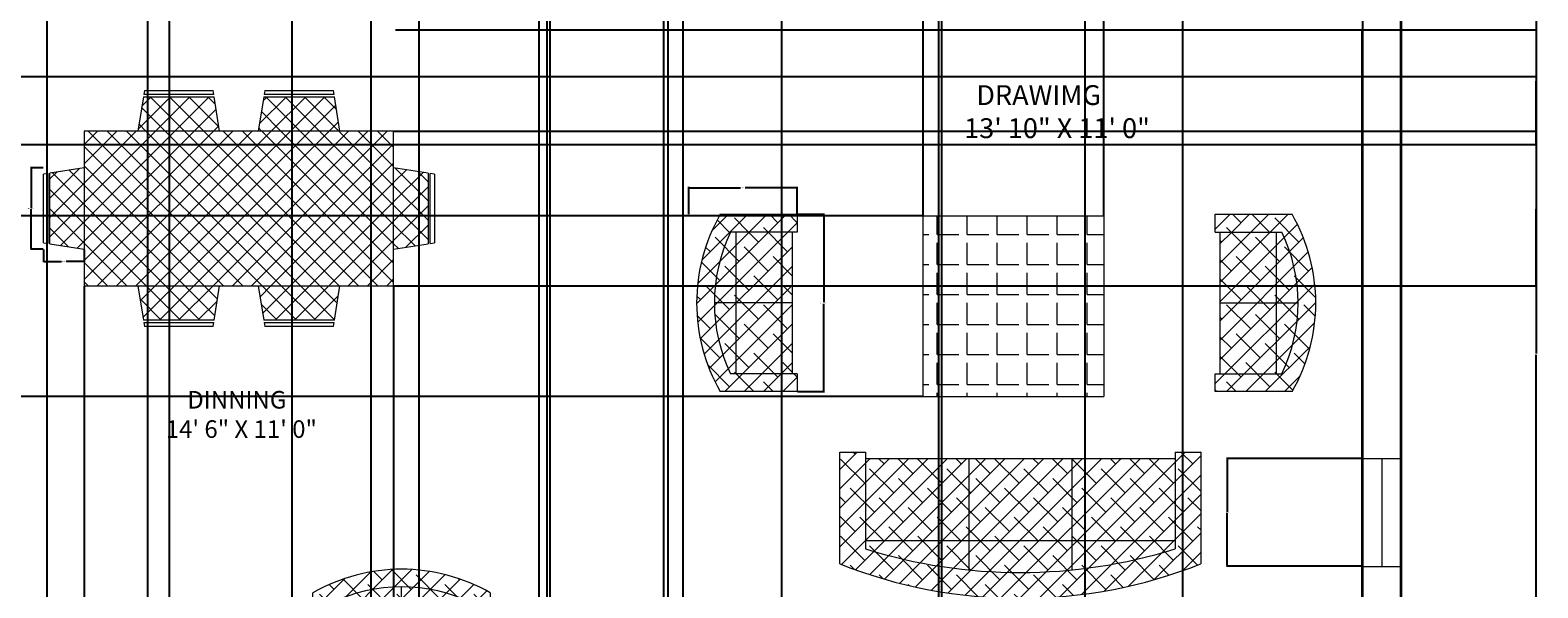
# Model space of a CAD drawing. Units: inches. Extents: x 2284228 to 3635239, y 3024422 to 8351872.
# Tile 4 of 7: x 3634888 to 3635239, y 8351470 to 8351600. Entities that reach past the tile are written whole.
import ezdxf

# ---------------------------------------------------------------- set-up
doc = ezdxf.new("R2010")
doc.units = ezdxf.units.IN
for name, color, linetype, lineweight in [('A-ANNO-DIMS', 2, 'Continuous', 18), ('A-AREA-IDEN', 7, 'Continuous', 18), ('A-FURN', 8, 'Continuous', 18), ('A-FURN-PATT', 9, 'Continuous', 13), ('A-GLAZ', 4, 'Continuous', 18), ('A-WALL', 7, 'Continuous', 35)]:
    doc.layers.add(name, color=color, linetype=linetype, lineweight=lineweight)
doc.styles.get("Standard").update_dxf_attribs({"font": 'arial.ttf'})
doc.dimstyles.get("Standard").update_dxf_attribs({"dimtxt": 0.18, "dimasz": 0.18, "dimexe": 0.18, "dimexo": 0.0625, "dimgap": 0.09, "dimtad": 0, "dimtih": 1, "dimtoh": 1, "dimdec": 4, "dimzin": 0, "dimdsep": 46, "dimtxsty": 'Standard', "dimcen": 0.09, "dimadec": 0, "dimazin": 0, "dimtfac": 1, "dimtdec": 4, "dimtofl": 0, "dimtmove": 0, "dimatfit": 3, "dimfxl": 1, "dimtolj": 1, "dimtzin": 0, "dimarcsym": 0})

# ---------------------------------------------------------------- blocks, each defined once
blk = doc.blocks.new('Sofa - Roundback 7 ft.')
for p, q in [((-12.00002, -32.4421), (-12.00003, -6.5971)), ((11.99997, -32.4421), (11.99998, -6.5971)), ((-36.000027, -34), (-36.000027, -11.4696)), ((-35.999844, -13.3819), (35.9998, -13.3819)), ((35.99998, -34), (35.99998, -11.4696)), ((-36.000027, -32.4421), (35.99998, -32.4421))]:
    blk.add_line(p, q)
for points in [[(-36.000027, -34), (-42.000027, -34), (-42.000027, -8)], [(41.99998, -8), (41.99998, -34), (35.99998, -34)]]:
    blk.add_lwpolyline(points)
for centre, radius, start, end in [((0, -114.25), 114.25, 68.43141, 111.5686), ((-0.00001, -127.1968), 121.1968, 72.72033, 107.2797)]:
    blk.add_arc(centre, radius, start, end)
blk = doc.blocks.new('Sofa - Roundback Loveseat 5 ft.')
for p, q in [((0, -32.44198), (0, -5.99998)), ((-24, -33.99998), (-24, -11.46958)), ((-23.9998, -13.38178), (23.99986, -13.38178)), ((24.00004, -33.99998), (24.00004, -11.46958)), ((-24, -32.44198), (24.00004, -32.44198))]:
    blk.add_line(p, q)
for points in [[(-24, -33.99998), (-30, -33.99998), (-30, -7.99998)], [(30.00004, -7.99998), (30.00004, -33.99998), (24.00004, -33.99998)]]:
    blk.add_lwpolyline(points)
for centre, radius, start, end in [((0, -60.24998), 60.24998, 60.13715, 119.8628), ((0, -61.38438), 55.38444, 64.32083, 115.6792)]:
    blk.add_arc(centre, radius, start, end)
blk = doc.blocks.new('CHAIR-DINING')
for p, q in [((1.25, 8), (0, 0)), ((1.25, 8), (17.72, 8)), ((1.48, 9.5), (1.33, 8.5)), ((17.64, 8.5), (1.33, 8.5)), ((1.48, 9.5), (17.48, 9.5)), ((17.64, 8.5), (17.48, 9.5)), ((18.97, 0), (17.72, 8))]:
    blk.add_line(p, q)
blk = doc.blocks.new('*D24')
at = {"layer": 'A-ANNO-DIMS', "color": 0, "lineweight": -2, "transparency": 16777216}
for p, q in [((3635066.29, 8351557.1), (3635072.6, 8351557.1)), ((3635072.42, 8351556.92), (3635072.42, 8351536.66)), ((3635072.42, 8351516.02), (3635072.42, 8351536.29)), ((3635066.29, 8351515.84), (3635072.6, 8351515.84))]:
    blk.add_line(p, q, dxfattribs=at)
at = {"layer": 'A-ANNO-DIMS', "color": 0, "transparency": 16777216}
for points in [[(3635072.39, 8351556.92), (3635072.45, 8351556.92), (3635072.42, 8351557.1)], [(3635072.39, 8351516.02), (3635072.45, 8351516.02), (3635072.42, 8351515.84)]]:
    blk.add_solid(points, dxfattribs=at)
at = {"layer": 'Defpoints', "color": 0, "transparency": 16777216}
for p in [(3635066.23, 8351557.1), (3635072.42, 8351557.1), (3635066.23, 8351515.84)]:
    blk.add_point(p, dxfattribs=at)
at = {"layer": 'A-ANNO-DIMS', "color": 0, "transparency": 16777216, "insert": (3635072.42, 8351536.47), "char_height": 0.18, "attachment_point": 5}
blk.add_mtext('\\A1;LOVESEAT 41 TYP.', dxfattribs=at)
blk = doc.blocks.new('*D25')
at = {"layer": 'A-ANNO-DIMS', "color": 0, "lineweight": -2, "transparency": 16777216}
for p, q in [((3635041.02, 8351557.16), (3635041.02, 8351563.47)), ((3635041.2, 8351563.29), (3635053.09, 8351563.29)), ((3635066.05, 8351563.29), (3635054.15, 8351563.29)), ((3635066.23, 8351557.16), (3635066.23, 8351563.47))]:
    blk.add_line(p, q, dxfattribs=at)
at = {"layer": 'A-ANNO-DIMS', "color": 0, "transparency": 16777216}
for points in [[(3635041.2, 8351563.32), (3635041.2, 8351563.26), (3635041.02, 8351563.29)], [(3635066.05, 8351563.32), (3635066.05, 8351563.26), (3635066.23, 8351563.29)]]:
    blk.add_solid(points, dxfattribs=at)
at = {"layer": 'Defpoints', "color": 0, "transparency": 16777216}
for p in [(3635041.02, 8351563.29), (3635041.02, 8351557.1), (3635066.23, 8351557.1)]:
    blk.add_point(p, dxfattribs=at)
at = {"layer": 'A-ANNO-DIMS', "color": 0, "transparency": 16777216, "insert": (3635053.62, 8351563.29), "char_height": 0.18, "attachment_point": 5}
blk.add_mtext('\\A1;25 TYP.', dxfattribs=at)
blk = doc.blocks.new('*D26')
at = {"layer": 'A-ANNO-DIMS', "color": 0, "lineweight": -2, "transparency": 16777216}
for p, q in [((3634890.78, 8351567.93), (3634887.82, 8351567.93)), ((3634888, 8351567.75), (3634888, 8351558.63)), ((3634888, 8351549.14), (3634888, 8351558.27)), ((3634890.79, 8351548.96), (3634887.82, 8351548.96))]:
    blk.add_line(p, q, dxfattribs=at)
at = {"layer": 'A-ANNO-DIMS', "color": 0, "transparency": 16777216}
for points in [[(3634888.03, 8351567.75), (3634887.97, 8351567.75), (3634888, 8351567.93)], [(3634888.03, 8351549.14), (3634887.97, 8351549.14), (3634888, 8351548.96)]]:
    blk.add_solid(points, dxfattribs=at)
at = {"layer": 'Defpoints', "color": 0, "transparency": 16777216}
for p in [(3634888, 8351567.93), (3634890.85, 8351567.93), (3634890.85, 8351548.96)]:
    blk.add_point(p, dxfattribs=at)
at = {"layer": 'A-ANNO-DIMS', "color": 0, "transparency": 16777216, "insert": (3634888, 8351558.45), "char_height": 0.18, "attachment_point": 5}
blk.add_mtext('\\A1;CHAIR 19 TYP.', dxfattribs=at)
blk = doc.blocks.new('*D27')
at = {"layer": 'A-ANNO-DIMS', "color": 0, "lineweight": -2, "transparency": 16777216}
for p, q in [((3634890.85, 8351548.9), (3634890.85, 8351545.94)), ((3634900.35, 8351548.9), (3634900.35, 8351545.94)), ((3634891.03, 8351546.12), (3634895.08, 8351546.12)), ((3634900.17, 8351546.12), (3634896.12, 8351546.12))]:
    blk.add_line(p, q, dxfattribs=at)
at = {"layer": 'A-ANNO-DIMS', "color": 0, "transparency": 16777216}
for points in [[(3634891.03, 8351546.15), (3634891.03, 8351546.09), (3634890.85, 8351546.12)], [(3634900.17, 8351546.15), (3634900.17, 8351546.09), (3634900.35, 8351546.12)]]:
    blk.add_solid(points, dxfattribs=at)
at = {"layer": 'Defpoints', "color": 0, "transparency": 16777216}
for p in [(3634890.85, 8351548.96), (3634900.35, 8351548.97), (3634890.85, 8351546.12)]:
    blk.add_point(p, dxfattribs=at)
at = {"layer": 'A-ANNO-DIMS', "color": 0, "transparency": 16777216, "insert": (3634895.6, 8351546.12), "char_height": 0.18, "attachment_point": 5}
blk.add_mtext('\\A1;10 TYP.', dxfattribs=at)
blk = doc.blocks.new('*D41')
at = {"layer": 'A-ANNO-DIMS', "color": 0, "lineweight": -2, "transparency": 16777216}
for p, q in [((3635053.81, 8351799.01), (3635238.38, 8351799.01)), ((3635238.2, 8351798.83), (3635238.2, 8351524.72)), ((3635238.2, 8351250.24), (3635238.2, 8351524.36)), ((3635039.81, 8351250.06), (3635238.38, 8351250.06))]:
    blk.add_line(p, q, dxfattribs=at)
at = {"layer": 'A-ANNO-DIMS', "color": 0, "transparency": 16777216}
for points in [[(3635238.17, 8351798.83), (3635238.23, 8351798.83), (3635238.2, 8351799.01)], [(3635238.17, 8351250.24), (3635238.23, 8351250.24), (3635238.2, 8351250.06)]]:
    blk.add_solid(points, dxfattribs=at)
at = {"layer": 'Defpoints', "color": 0, "transparency": 16777216}
for p in [(3635053.75, 8351799.01), (3635238.2, 8351799.01), (3635039.75, 8351250.06)]:
    blk.add_point(p, dxfattribs=at)
at = {"layer": 'A-ANNO-DIMS', "color": 0, "transparency": 16777216, "insert": (3635238.2, 8351524.54), "char_height": 0.18, "attachment_point": 5}
blk.add_mtext('\\A1;549', dxfattribs=at)
blk = doc.blocks.new('*D49')
at = {"layer": 'A-ANNO-DIMS', "color": 0, "lineweight": -2, "transparency": 16777216}
for p, q in [((3634891.75, 8351310.63), (3634891.75, 8351830.64)), ((3634891.93, 8351830.46), (3634965.47, 8351830.46)), ((3635039.57, 8351830.46), (3634966.03, 8351830.46)), ((3635039.75, 8351310.63), (3635039.75, 8351830.64))]:
    blk.add_line(p, q, dxfattribs=at)
at = {"layer": 'A-ANNO-DIMS', "color": 0, "transparency": 16777216}
for points in [[(3634891.93, 8351830.49), (3634891.93, 8351830.43), (3634891.75, 8351830.46)], [(3635039.57, 8351830.49), (3635039.57, 8351830.43), (3635039.75, 8351830.46)]]:
    blk.add_solid(points, dxfattribs=at)
at = {"layer": 'Defpoints', "color": 0, "transparency": 16777216}
for p in [(3635039.75, 8351830.46), (3634891.75, 8351310.56), (3635039.75, 8351310.56)]:
    blk.add_point(p, dxfattribs=at)
at = {"layer": 'A-ANNO-DIMS', "color": 0, "transparency": 16777216, "insert": (3634965.75, 8351830.46), "char_height": 0.18, "attachment_point": 5}
blk.add_mtext('\\A1;148', dxfattribs=at)
blk = doc.blocks.new('*D52')
at = {"layer": 'A-ANNO-DIMS', "color": 0, "lineweight": -2, "transparency": 16777216}
for p, q in [((3635099.83, 8351748.5), (3635099.83, 8351218.43)), ((3635155.88, 8351748.5), (3635155.88, 8351218.43)), ((3635100.01, 8351218.61), (3635127.46, 8351218.61)), ((3635155.7, 8351218.61), (3635128.25, 8351218.61))]:
    blk.add_line(p, q, dxfattribs=at)
at = {"layer": 'A-ANNO-DIMS', "color": 0, "transparency": 16777216}
for points in [[(3635100.01, 8351218.64), (3635100.01, 8351218.58), (3635099.83, 8351218.61)], [(3635155.7, 8351218.64), (3635155.7, 8351218.58), (3635155.88, 8351218.61)]]:
    blk.add_solid(points, dxfattribs=at)
at = {"layer": 'Defpoints', "color": 0, "transparency": 16777216}
for p in [(3635099.83, 8351748.56), (3635155.88, 8351748.56), (3635155.88, 8351218.61)]:
    blk.add_point(p, dxfattribs=at)
at = {"layer": 'A-ANNO-DIMS', "color": 0, "transparency": 16777216, "insert": (3635127.85, 8351218.61), "char_height": 0.18, "attachment_point": 5}
blk.add_mtext('\\A1;56.06', dxfattribs=at)
blk = doc.blocks.new('*D53')
at = {"layer": 'A-ANNO-DIMS', "color": 0, "lineweight": -2, "transparency": 16777216}
for p, q in [((3635155.88, 8351748.5), (3635155.88, 8351218.43)), ((3635197.75, 8351748.5), (3635197.75, 8351218.43)), ((3635156.06, 8351218.61), (3635176.42, 8351218.61)), ((3635197.57, 8351218.61), (3635177.21, 8351218.61))]:
    blk.add_line(p, q, dxfattribs=at)
at = {"layer": 'A-ANNO-DIMS', "color": 0, "transparency": 16777216}
for points in [[(3635156.06, 8351218.64), (3635156.06, 8351218.58), (3635155.88, 8351218.61)], [(3635197.57, 8351218.64), (3635197.57, 8351218.58), (3635197.75, 8351218.61)]]:
    blk.add_solid(points, dxfattribs=at)
at = {"layer": 'Defpoints', "color": 0, "transparency": 16777216}
for p in [(3635155.88, 8351748.56), (3635197.75, 8351748.56), (3635197.75, 8351218.61)]:
    blk.add_point(p, dxfattribs=at)
at = {"layer": 'A-ANNO-DIMS', "color": 0, "transparency": 16777216, "insert": (3635176.82, 8351218.61), "char_height": 0.18, "attachment_point": 5}
blk.add_mtext('\\A1;41.87', dxfattribs=at)
blk = doc.blocks.new('*D54')
at = {"layer": 'A-ANNO-DIMS', "color": 0, "lineweight": -2, "transparency": 16777216}
for p, q in [((3635006.17, 8351652.5), (3635006.17, 8351218.43)), ((3635036.17, 8351652.5), (3635036.17, 8351218.43)), ((3635006.35, 8351218.61), (3635020.95, 8351218.61)), ((3635035.99, 8351218.61), (3635021.38, 8351218.61))]:
    blk.add_line(p, q, dxfattribs=at)
at = {"layer": 'A-ANNO-DIMS', "color": 0, "transparency": 16777216}
for points in [[(3635006.35, 8351218.64), (3635006.35, 8351218.58), (3635006.17, 8351218.61)], [(3635035.99, 8351218.64), (3635035.99, 8351218.58), (3635036.17, 8351218.61)]]:
    blk.add_solid(points, dxfattribs=at)
at = {"layer": 'Defpoints', "color": 0, "transparency": 16777216}
for p in [(3635006.17, 8351652.56), (3635036.17, 8351652.56), (3635036.17, 8351218.61)]:
    blk.add_point(p, dxfattribs=at)
at = {"layer": 'A-ANNO-DIMS', "color": 0, "transparency": 16777216, "insert": (3635021.17, 8351218.61), "char_height": 0.18, "attachment_point": 5}
blk.add_mtext('\\A1;30', dxfattribs=at)
blk = doc.blocks.new('*D57')
at = {"layer": 'A-ANNO-DIMS', "color": 0, "lineweight": -2, "transparency": 16777216}
for p, q in [((3635035.25, 8351378.63), (3635035.25, 8351830.64)), ((3635035.43, 8351830.46), (3635048.63, 8351830.46)), ((3635062.47, 8351830.46), (3635049.28, 8351830.46)), ((3635062.65, 8351378.63), (3635062.65, 8351830.64))]:
    blk.add_line(p, q, dxfattribs=at)
at = {"layer": 'A-ANNO-DIMS', "color": 0, "transparency": 16777216}
for points in [[(3635035.43, 8351830.49), (3635035.43, 8351830.43), (3635035.25, 8351830.46)], [(3635062.47, 8351830.49), (3635062.47, 8351830.43), (3635062.65, 8351830.46)]]:
    blk.add_solid(points, dxfattribs=at)
at = {"layer": 'Defpoints', "color": 0, "transparency": 16777216}
for p in [(3635062.65, 8351830.46), (3635035.25, 8351378.57), (3635062.65, 8351378.57)]:
    blk.add_point(p, dxfattribs=at)
at = {"layer": 'A-ANNO-DIMS', "color": 0, "transparency": 16777216, "insert": (3635048.95, 8351830.46), "char_height": 0.18, "attachment_point": 5}
blk.add_mtext('\\A1;27.4', dxfattribs=at)
blk = doc.blocks.new('*D59')
at = {"layer": 'A-ANNO-DIMS', "color": 0, "lineweight": -2, "transparency": 16777216}
for p, q in [((3635099.24, 8351408.73), (3635099.24, 8351830.64)), ((3635099.42, 8351830.46), (3635115.78, 8351830.46)), ((3635133.07, 8351830.46), (3635116.71, 8351830.46)), ((3635133.25, 8351408.73), (3635133.25, 8351830.64))]:
    blk.add_line(p, q, dxfattribs=at)
at = {"layer": 'A-ANNO-DIMS', "color": 0, "transparency": 16777216}
for points in [[(3635099.42, 8351830.49), (3635099.42, 8351830.43), (3635099.24, 8351830.46)], [(3635133.07, 8351830.49), (3635133.07, 8351830.43), (3635133.25, 8351830.46)]]:
    blk.add_solid(points, dxfattribs=at)
at = {"layer": 'Defpoints', "color": 0, "transparency": 16777216}
for p in [(3635133.25, 8351830.46), (3635099.24, 8351408.67), (3635133.25, 8351408.67)]:
    blk.add_point(p, dxfattribs=at)
at = {"layer": 'A-ANNO-DIMS', "color": 0, "transparency": 16777216, "insert": (3635116.24, 8351830.46), "char_height": 0.18, "attachment_point": 5}
blk.add_mtext('\\A1;34.016', dxfattribs=at)
blk = doc.blocks.new('*D65')
at = {"layer": 'A-ANNO-DIMS', "color": 0, "lineweight": -2, "transparency": 16777216}
for p, q in [((3634900.35, 8351540.39), (3634900.35, 8351218.43)), ((3634972.35, 8351540.39), (3634972.35, 8351218.43)), ((3634900.53, 8351218.61), (3634936.13, 8351218.61)), ((3634972.17, 8351218.61), (3634936.57, 8351218.61))]:
    blk.add_line(p, q, dxfattribs=at)
at = {"layer": 'A-ANNO-DIMS', "color": 0, "transparency": 16777216}
for points in [[(3634900.53, 8351218.64), (3634900.53, 8351218.58), (3634900.35, 8351218.61)], [(3634972.17, 8351218.64), (3634972.17, 8351218.58), (3634972.35, 8351218.61)]]:
    blk.add_solid(points, dxfattribs=at)
at = {"layer": 'Defpoints', "color": 0, "transparency": 16777216}
for p in [(3634900.35, 8351540.45), (3634972.35, 8351540.45), (3634972.35, 8351218.61)]:
    blk.add_point(p, dxfattribs=at)
at = {"layer": 'A-ANNO-DIMS', "color": 0, "transparency": 16777216, "insert": (3634936.35, 8351218.61), "char_height": 0.18, "attachment_point": 5}
blk.add_mtext('\\A1;72', dxfattribs=at)
blk = doc.blocks.new('*D66')
at = {"layer": 'A-ANNO-DIMS', "color": 0, "lineweight": -2, "transparency": 16777216}
for p, q in [((3634972.41, 8351576.45), (3635238.38, 8351576.45)), ((3635238.2, 8351576.27), (3635238.2, 8351558.63)), ((3635238.2, 8351540.63), (3635238.2, 8351558.27)), ((3634972.41, 8351540.45), (3635238.38, 8351540.45))]:
    blk.add_line(p, q, dxfattribs=at)
at = {"layer": 'A-ANNO-DIMS', "color": 0, "transparency": 16777216}
for points in [[(3635238.17, 8351576.27), (3635238.23, 8351576.27), (3635238.2, 8351576.45)], [(3635238.17, 8351540.63), (3635238.23, 8351540.63), (3635238.2, 8351540.45)]]:
    blk.add_solid(points, dxfattribs=at)
at = {"layer": 'Defpoints', "color": 0, "transparency": 16777216}
for p in [(3634972.35, 8351576.45), (3635238.2, 8351576.45), (3634972.35, 8351540.45)]:
    blk.add_point(p, dxfattribs=at)
at = {"layer": 'A-ANNO-DIMS', "color": 0, "transparency": 16777216, "insert": (3635238.2, 8351558.45), "char_height": 0.18, "attachment_point": 5}
blk.add_mtext('\\A1;36', dxfattribs=at)
blk = doc.blocks.new('*D67')
at = {"layer": 'A-ANNO-DIMS', "color": 0, "lineweight": -2, "transparency": 16777216}
for p, q in [((3634972.81, 8351600.06), (3635238.38, 8351600.06)), ((3635238.2, 8351599.88), (3635238.2, 8351588.44)), ((3635238.2, 8351576.63), (3635238.2, 8351588.08)), ((3634972.41, 8351576.45), (3635238.38, 8351576.45))]:
    blk.add_line(p, q, dxfattribs=at)
at = {"layer": 'A-ANNO-DIMS', "color": 0, "transparency": 16777216}
for points in [[(3635238.17, 8351599.88), (3635238.23, 8351599.88), (3635238.2, 8351600.06)], [(3635238.17, 8351576.63), (3635238.23, 8351576.63), (3635238.2, 8351576.45)]]:
    blk.add_solid(points, dxfattribs=at)
at = {"layer": 'Defpoints', "color": 0, "transparency": 16777216}
for p in [(3634972.75, 8351600.06), (3635238.2, 8351600.06), (3634972.35, 8351576.45)]:
    blk.add_point(p, dxfattribs=at)
at = {"layer": 'A-ANNO-DIMS', "color": 0, "transparency": 16777216, "insert": (3635238.2, 8351588.26), "char_height": 0.18, "attachment_point": 5}
blk.add_mtext('\\A1;23.61', dxfattribs=at)
blk = doc.blocks.new('*D69')
at = {"layer": 'A-ANNO-DIMS', "color": 0, "lineweight": -2, "transparency": 16777216}
for p, q in [((3634752.31, 8351589.14), (3635238.38, 8351589.14)), ((3635238.2, 8351588.96), (3635238.2, 8351581.41)), ((3635238.2, 8351573.51), (3635238.2, 8351581.05)), ((3634752.31, 8351573.33), (3635238.38, 8351573.33))]:
    blk.add_line(p, q, dxfattribs=at)
at = {"layer": 'A-ANNO-DIMS', "color": 0, "transparency": 16777216}
for points in [[(3635238.17, 8351588.96), (3635238.23, 8351588.96), (3635238.2, 8351589.14)], [(3635238.17, 8351573.51), (3635238.23, 8351573.51), (3635238.2, 8351573.33)]]:
    blk.add_solid(points, dxfattribs=at)
at = {"layer": 'Defpoints', "color": 0, "transparency": 16777216}
for p in [(3634752.25, 8351589.14), (3635238.2, 8351589.14), (3634752.25, 8351573.33)]:
    blk.add_point(p, dxfattribs=at)
at = {"layer": 'A-ANNO-DIMS', "color": 0, "transparency": 16777216, "insert": (3635238.2, 8351581.23), "char_height": 0.18, "attachment_point": 5}
blk.add_mtext('\\A1;15.813', dxfattribs=at)
blk = doc.blocks.new('*D71')
at = {"layer": 'A-ANNO-DIMS', "color": 0, "lineweight": -2, "transparency": 16777216}
for p, q in [((3635197.69, 8351500.24), (3635166.12, 8351500.24)), ((3635166.3, 8351500.06), (3635166.3, 8351487.89)), ((3635166.3, 8351475.36), (3635166.3, 8351487.52)), ((3635197.69, 8351475.18), (3635166.12, 8351475.18))]:
    blk.add_line(p, q, dxfattribs=at)
at = {"layer": 'A-ANNO-DIMS', "color": 0, "transparency": 16777216}
for points in [[(3635166.27, 8351500.06), (3635166.33, 8351500.06), (3635166.3, 8351500.24)], [(3635166.27, 8351475.36), (3635166.33, 8351475.36), (3635166.3, 8351475.18)]]:
    blk.add_solid(points, dxfattribs=at)
at = {"layer": 'Defpoints', "color": 0, "transparency": 16777216}
for p in [(3635166.3, 8351500.24), (3635197.75, 8351500.24), (3635197.75, 8351475.18)]:
    blk.add_point(p, dxfattribs=at)
at = {"layer": 'A-ANNO-DIMS', "color": 0, "transparency": 16777216, "insert": (3635166.3, 8351487.71), "char_height": 0.18, "attachment_point": 5}
blk.add_mtext('\\A1;25.06', dxfattribs=at)
blk = doc.blocks.new('*D74')
at = {"layer": 'A-ANNO-DIMS', "color": 0, "lineweight": -2, "transparency": 16777216}
for p, q in [((3634920.21, 8351331.63), (3634920.21, 8351830.64)), ((3634920.39, 8351830.46), (3634948.84, 8351830.46)), ((3634978.09, 8351830.46), (3634949.63, 8351830.46)), ((3634978.27, 8351331.63), (3634978.27, 8351830.64))]:
    blk.add_line(p, q, dxfattribs=at)
at = {"layer": 'A-ANNO-DIMS', "color": 0, "transparency": 16777216}
for points in [[(3634920.39, 8351830.49), (3634920.39, 8351830.43), (3634920.21, 8351830.46)], [(3634978.09, 8351830.49), (3634978.09, 8351830.43), (3634978.27, 8351830.46)]]:
    blk.add_solid(points, dxfattribs=at)
at = {"layer": 'Defpoints', "color": 0, "transparency": 16777216}
for p in [(3634978.27, 8351830.46), (3634920.21, 8351331.56), (3634978.27, 8351331.56)]:
    blk.add_point(p, dxfattribs=at)
at = {"layer": 'A-ANNO-DIMS', "color": 0, "transparency": 16777216, "insert": (3634949.24, 8351830.46), "char_height": 0.18, "attachment_point": 5}
blk.add_mtext('\\A1;58.06', dxfattribs=at)
blk = doc.blocks.new('*D78')
at = {"layer": 'A-ANNO-DIMS', "color": 0, "lineweight": -2, "transparency": 16777216}
for p, q in [((3635095.59, 8351556.78), (3635095.59, 8351830.64)), ((3635095.77, 8351830.46), (3635116.37, 8351830.46)), ((3635137.41, 8351830.46), (3635116.81, 8351830.46)), ((3635137.59, 8351556.78), (3635137.59, 8351830.64))]:
    blk.add_line(p, q, dxfattribs=at)
at = {"layer": 'A-ANNO-DIMS', "color": 0, "transparency": 16777216}
for points in [[(3635095.77, 8351830.49), (3635095.77, 8351830.43), (3635095.59, 8351830.46)], [(3635137.41, 8351830.49), (3635137.41, 8351830.43), (3635137.59, 8351830.46)]]:
    blk.add_solid(points, dxfattribs=at)
at = {"layer": 'Defpoints', "color": 0, "transparency": 16777216}
for p in [(3635137.59, 8351830.46), (3635095.59, 8351556.72), (3635137.59, 8351556.72)]:
    blk.add_point(p, dxfattribs=at)
at = {"layer": 'A-ANNO-DIMS', "color": 0, "transparency": 16777216, "insert": (3635116.59, 8351830.46), "char_height": 0.18, "attachment_point": 5}
blk.add_mtext('\\A1;42', dxfattribs=at)
blk = doc.blocks.new('*D79')
at = {"layer": 'A-ANNO-DIMS', "color": 0, "lineweight": -2, "transparency": 16777216}
for p, q in [((3635095.53, 8351556.72), (3634669.29, 8351556.72)), ((3634669.47, 8351556.54), (3634669.47, 8351535.9)), ((3634669.47, 8351514.9), (3634669.47, 8351535.54)), ((3635095.53, 8351514.72), (3634669.29, 8351514.72))]:
    blk.add_line(p, q, dxfattribs=at)
at = {"layer": 'A-ANNO-DIMS', "color": 0, "transparency": 16777216}
for points in [[(3634669.44, 8351556.54), (3634669.5, 8351556.54), (3634669.47, 8351556.72)], [(3634669.44, 8351514.9), (3634669.5, 8351514.9), (3634669.47, 8351514.72)]]:
    blk.add_solid(points, dxfattribs=at)
at = {"layer": 'Defpoints', "color": 0, "transparency": 16777216}
for p in [(3634669.47, 8351556.72), (3635095.59, 8351556.72), (3635095.59, 8351514.72)]:
    blk.add_point(p, dxfattribs=at)
at = {"layer": 'A-ANNO-DIMS', "color": 0, "transparency": 16777216, "insert": (3634669.47, 8351535.72), "char_height": 0.18, "attachment_point": 5}
blk.add_mtext('\\A1;42', dxfattribs=at)
blk = doc.blocks.new('*D80')
at = {"layer": 'A-ANNO-DIMS', "color": 0, "lineweight": -2, "transparency": 16777216}
for p, q in [((3634948.75, 8351437.56), (3634948.75, 8351830.64)), ((3634948.93, 8351830.46), (3634978.53, 8351830.46)), ((3635008.57, 8351830.46), (3634978.97, 8351830.46)), ((3635008.75, 8351437.56), (3635008.75, 8351830.64))]:
    blk.add_line(p, q, dxfattribs=at)
at = {"layer": 'A-ANNO-DIMS', "color": 0, "transparency": 16777216}
for points in [[(3634948.93, 8351830.49), (3634948.93, 8351830.43), (3634948.75, 8351830.46)], [(3635008.57, 8351830.49), (3635008.57, 8351830.43), (3635008.75, 8351830.46)]]:
    blk.add_solid(points, dxfattribs=at)
at = {"layer": 'Defpoints', "color": 0, "transparency": 16777216}
for p in [(3635008.75, 8351830.46), (3634948.75, 8351437.49), (3635008.75, 8351437.49)]:
    blk.add_point(p, dxfattribs=at)
at = {"layer": 'A-ANNO-DIMS', "color": 0, "transparency": 16777216, "insert": (3634978.75, 8351830.46), "char_height": 0.18, "attachment_point": 5}
blk.add_mtext('\\A1;60', dxfattribs=at)
blk = doc.blocks.new('*D82')
at = {"layer": 'A-ANNO-DIMS', "color": 0, "lineweight": -2, "transparency": 16777216}
for p, q in [((3634915.11, 8351783.43), (3634915.11, 8351218.43)), ((3634967.04, 8351783.43), (3634967.04, 8351218.43)), ((3634915.29, 8351218.61), (3634940.68, 8351218.61)), ((3634966.86, 8351218.61), (3634941.47, 8351218.61))]:
    blk.add_line(p, q, dxfattribs=at)
at = {"layer": 'A-ANNO-DIMS', "color": 0, "transparency": 16777216}
for points in [[(3634915.29, 8351218.64), (3634915.29, 8351218.58), (3634915.11, 8351218.61)], [(3634966.86, 8351218.64), (3634966.86, 8351218.58), (3634967.04, 8351218.61)]]:
    blk.add_solid(points, dxfattribs=at)
at = {"layer": 'Defpoints', "color": 0, "transparency": 16777216}
for p in [(3634915.11, 8351783.5), (3634967.04, 8351783.5), (3634967.04, 8351218.61)]:
    blk.add_point(p, dxfattribs=at)
at = {"layer": 'A-ANNO-DIMS', "color": 0, "transparency": 16777216, "insert": (3634941.08, 8351218.61), "char_height": 0.18, "attachment_point": 5}
blk.add_mtext('\\A1;51.94', dxfattribs=at)
blk = doc.blocks.new('*D83')
at = {"layer": 'A-ANNO-DIMS', "color": 0, "lineweight": -2, "transparency": 16777216}
for p, q in [((3634967.04, 8351783.43), (3634967.04, 8351218.43)), ((3635008.03, 8351783.43), (3635008.03, 8351218.43)), ((3634967.22, 8351218.61), (3634987.14, 8351218.61)), ((3635007.85, 8351218.61), (3634987.93, 8351218.61))]:
    blk.add_line(p, q, dxfattribs=at)
at = {"layer": 'A-ANNO-DIMS', "color": 0, "transparency": 16777216}
for points in [[(3634967.22, 8351218.64), (3634967.22, 8351218.58), (3634967.04, 8351218.61)], [(3635007.85, 8351218.64), (3635007.85, 8351218.58), (3635008.03, 8351218.61)]]:
    blk.add_solid(points, dxfattribs=at)
at = {"layer": 'Defpoints', "color": 0, "transparency": 16777216}
for p in [(3634967.04, 8351783.5), (3635008.03, 8351783.5), (3635008.03, 8351218.61)]:
    blk.add_point(p, dxfattribs=at)
at = {"layer": 'A-ANNO-DIMS', "color": 0, "transparency": 16777216, "insert": (3634987.54, 8351218.61), "char_height": 0.18, "attachment_point": 5}
blk.add_mtext('\\A1;40.98', dxfattribs=at)

msp = doc.modelspace()

# ---------------------------------------------------------------- hatches: boundary and pattern name
at = {"layer": 'A-FURN-PATT'}
h = msp.add_hatch(dxfattribs=at)
h.set_pattern_fill('ANSI37', color=256)
h.paths.add_polyline_path([(3634930.5828, 8351584.4517), (3634914.1141, 8351584.4517), (3634912.8641, 8351576.4517), (3634931.8329, 8351576.4517)])
h.paths.add_polyline_path([(3634958.5828, 8351584.4517), (3634942.1141, 8351584.4517), (3634940.8641, 8351576.4517), (3634959.8329, 8351576.4517)])
h.paths.add_polyline_path([(3634900.3485, 8351567.9361), (3634892.3485, 8351566.6861), (3634892.3485, 8351550.2173), (3634900.3485, 8351548.9673)])
h.paths.add_polyline_path([(3634980.3485, 8351566.6861), (3634972.3485, 8351567.9361), (3634972.3485, 8351548.9673), (3634980.3485, 8351550.2173)])
h.paths.add_polyline_path([(3634959.8329, 8351540.4517), (3634940.8641, 8351540.4517), (3634942.1141, 8351532.4517), (3634958.5828, 8351532.4517)])
h.paths.add_polyline_path([(3634931.8329, 8351540.4517), (3634912.8641, 8351540.4517), (3634914.1141, 8351532.4517), (3634930.5828, 8351532.4517)])
h = msp.add_hatch(dxfattribs=at)
h.set_pattern_fill('ANSI37', color=256)
h.paths.add_polyline_path([(3634972.3485, 8351576.4517), (3634900.3485, 8351576.4517), (3634900.3485, 8351540.4517), (3634972.3485, 8351540.4517)])
h = msp.add_hatch(dxfattribs=at)
h.set_pattern_fill('ANSI38', color=256)
h.paths.add_polyline_path([(3634930.7271, 8351308.1081), (3634917.6211, 8351308.1081), (3634917.6211, 8351291.6054), (3634930.7271, 8351291.6054)], flags=17)
h.paths.add_polyline_path([(3634917.6211, 8351308.1081), (3634916.3066, 8351308.1081, 0.11251889), (3634912.5453, 8351291.6054), (3634917.6211, 8351291.6054)], flags=17)
h.paths.add_polyline_path([(3634930.7271, 8351291.6054), (3634917.6211, 8351291.6054), (3634917.6211, 8351275.1027), (3634930.7271, 8351275.1027)], flags=17)
h.paths.add_polyline_path([(3634917.6211, 8351291.6054), (3634912.5453, 8351291.6054, 0.11251869), (3634916.3066, 8351275.1027), (3634917.6211, 8351275.1027)], flags=17)
h.paths.add_polyline_path([(3634931.7984, 8351312.2337), (3634913.9206, 8351312.2337, 0.26666697), (3634913.9206, 8351270.977), (3634931.7984, 8351270.977), (3634931.7984, 8351275.1027), (3634916.3066, 8351275.1027, -0.11251869), (3634912.5453, 8351291.6054, -0.11251889), (3634916.3066, 8351308.1081), (3634931.7984, 8351308.1081)])
h.paths.add_polyline_path([(3635011.8389, 8351305.2814), (3634998.7329, 8351305.2814), (3634998.7329, 8351288.7787), (3635011.8389, 8351288.7787)], flags=17)
h.paths.add_polyline_path([(3635011.8389, 8351288.7787), (3634998.7329, 8351288.7787), (3634998.7329, 8351272.276), (3635011.8389, 8351272.276)], flags=17)
h.paths.add_polyline_path([(3635016.9148, 8351288.7787), (3635011.8389, 8351288.7787), (3635011.8389, 8351272.276), (3635013.1534, 8351272.276, 0.11251889)], flags=17)
h.paths.add_polyline_path([(3635013.1534, 8351305.2814), (3635011.8389, 8351305.2814), (3635011.8389, 8351288.7787), (3635016.9148, 8351288.7787, 0.11251869)], flags=17)
h.paths.add_polyline_path([(3635015.5395, 8351309.407), (3634997.6616, 8351309.407), (3634997.6616, 8351305.2814), (3635013.1534, 8351305.2814, -0.11251869), (3635016.9148, 8351288.7787, -0.11251889), (3635013.1534, 8351272.276), (3634997.6616, 8351272.276), (3634997.6616, 8351268.1503), (3635015.5395, 8351268.1503, 0.26666697)])
h.paths.add_polyline_path([(3635065.1595, 8351552.9755), (3635052.0535, 8351552.9755), (3635052.0535, 8351536.4728), (3635065.1595, 8351536.4728)], flags=17)
h.paths.add_polyline_path([(3635065.1595, 8351536.4728), (3635052.0535, 8351536.4728), (3635052.0535, 8351519.9701), (3635065.1595, 8351519.9701)], flags=17)
h.paths.add_polyline_path([(3635052.0535, 8351536.4728), (3635046.9776, 8351536.4728, 0.11251869), (3635050.739, 8351519.9701), (3635052.0535, 8351519.9701)], flags=17)
h.paths.add_polyline_path([(3635052.0535, 8351552.9755), (3635050.739, 8351552.9755, 0.11251889), (3635046.9776, 8351536.4728), (3635052.0535, 8351536.4728)], flags=17)
h.paths.add_polyline_path([(3635066.2308, 8351519.9701), (3635050.739, 8351519.9701, -0.11251869), (3635046.9776, 8351536.4728, -0.11251889), (3635050.739, 8351552.9755), (3635066.2308, 8351552.9755), (3635066.2308, 8351557.1011), (3635048.3529, 8351557.1011, 0.26666697), (3635048.3529, 8351515.8444), (3635066.2308, 8351515.8444)])
h.paths.add_polyline_path([(3635177.7039, 8351552.9754), (3635164.5979, 8351552.9754), (3635164.5979, 8351536.4728), (3635177.7039, 8351536.4728)], flags=17)
h.paths.add_polyline_path([(3635179.0184, 8351552.9754), (3635177.7039, 8351552.9754), (3635177.7039, 8351536.4728), (3635182.7797, 8351536.4728, 0.11251869)], flags=17)
h.paths.add_polyline_path([(3635177.7039, 8351536.4728), (3635164.5979, 8351536.4728), (3635164.5979, 8351519.9701), (3635177.7039, 8351519.9701)], flags=17)
h.paths.add_polyline_path([(3635182.7797, 8351536.4728), (3635177.7039, 8351536.4728), (3635177.7039, 8351519.9701), (3635179.0184, 8351519.9701, 0.11251889)], flags=17)
h.paths.add_polyline_path([(3635181.4045, 8351557.1011), (3635163.5266, 8351557.1011), (3635163.5266, 8351552.9754), (3635179.0184, 8351552.9754, -0.11251869), (3635182.7797, 8351536.4728, -0.11251889), (3635179.0184, 8351519.9701), (3635163.5266, 8351519.9701), (3635163.5266, 8351515.8444), (3635181.4045, 8351515.8444, 0.26666697)])
h.paths.add_polyline_path([(3635154.1523, 8351500.1911), (3635130.1523, 8351500.1911), (3635130.1523, 8351481.1309), (3635154.1523, 8351481.1309)], flags=17)
h.paths.add_polyline_path([(3635130.1523, 8351500.1911), (3635106.1523, 8351500.1911), (3635106.1523, 8351481.1309), (3635130.1523, 8351481.1309)], flags=17)
h.paths.add_polyline_path([(3635106.1523, 8351500.1911), (3635082.1523, 8351500.1911), (3635082.1523, 8351481.1309), (3635106.1523, 8351481.1309)], flags=17)
h.paths.add_polyline_path([(3635106.1523, 8351481.1309), (3635082.1523, 8351481.1309), (3635082.1523, 8351479.2191, 0.05064665), (3635106.1523, 8351474.3445)], flags=17)
h.paths.add_polyline_path([(3635130.1523, 8351481.1309), (3635106.1523, 8351481.1309), (3635106.1523, 8351474.3461), (3635106.1523, 8351474.3445, 0.04962821), (3635130.1523, 8351474.3445)], flags=17)
h.paths.add_polyline_path([(3635154.1523, 8351479.2191), (3635154.1523, 8351481.1309), (3635130.1523, 8351481.1309), (3635130.1523, 8351474.3445, 0.05064665)], flags=17)
h.paths.add_polyline_path([(3635160.1523, 8351475.749), (3635160.1523, 8351501.749), (3635154.1523, 8351501.749), (3635154.1523, 8351479.2191, -0.15194781), (3635082.1523, 8351479.2191), (3635082.1523, 8351501.749), (3635076.1523, 8351501.749), (3635076.1523, 8351475.749, 0.19047621)])
h = msp.add_hatch(dxfattribs=at)
h.set_pattern_fill('ANGLE', color=256)
h.set_pattern_definition([(0, (0, 0), (0, 6.985), [5.08, -1.905]), (90, (0, 0), (-6.985, 4e-16), [5.08, -1.905])])
h.paths.add_polyline_path([(3635137.5898, 8351556.7209), (3635095.5898, 8351556.7209), (3635095.5898, 8351514.7209), (3635137.5898, 8351514.7209)])
h = msp.add_hatch(dxfattribs=at)
h.set_pattern_fill('ANSI38', color=256)
h.paths.add_polyline_path([(3634933.1946, 8351444.2171), (3634914.1344, 8351444.2171), (3634914.1344, 8351420.2171), (3634933.1946, 8351420.2171)], flags=17)
h.paths.add_polyline_path([(3634933.1946, 8351420.2171), (3634914.1344, 8351420.2171), (3634914.1344, 8351396.2171), (3634933.1946, 8351396.2171)], flags=17)
h.paths.add_polyline_path([(3634933.1946, 8351396.2171), (3634914.1344, 8351396.2171), (3634914.1344, 8351372.2171), (3634933.1946, 8351372.2171)], flags=17)
h.paths.add_polyline_path([(3634914.1344, 8351396.2171), (3634907.348, 8351396.2171, 0.05064665), (3634912.2226, 8351372.2171), (3634914.1344, 8351372.2171)], flags=17)
h.paths.add_polyline_path([(3634914.1344, 8351420.2171), (3634907.348, 8351420.2171, 0.04962821), (3634907.348, 8351396.2171), (3634914.1344, 8351396.2171)], flags=17)
h.paths.add_polyline_path([(3634914.1344, 8351444.2171), (3634912.2226, 8351444.2171, 0.05064665), (3634907.348, 8351420.2171), (3634914.1344, 8351420.2171)], flags=17)
h.paths.add_polyline_path([(3634934.7525, 8351450.2171), (3634908.7525, 8351450.2171, 0.19047621), (3634908.7525, 8351366.2171), (3634934.7525, 8351366.2171), (3634934.7525, 8351372.2171), (3634912.2226, 8351372.2171, -0.05064665), (3634907.348, 8351396.2171, -0.10052754), (3634912.2226, 8351444.2171), (3634934.7525, 8351444.2171)])
h.paths.add_polyline_path([(3634993.654, 8351371.3187), (3634993.654, 8351389.1966), (3634989.5284, 8351389.1966), (3634989.5284, 8351373.7048, -0.22792319), (3634956.523, 8351373.7048), (3634956.523, 8351389.1966), (3634952.3973, 8351389.1966), (3634952.3973, 8351371.3187, 0.26666697)])
h.paths.add_polyline_path([(3634989.5284, 8351373.7048), (3634989.5284, 8351375.0193), (3634973.0257, 8351375.0193), (3634973.0257, 8351369.9434, 0.11251869)], flags=17)
h.paths.add_polyline_path([(3634973.0257, 8351375.0193), (3634956.523, 8351375.0193), (3634956.523, 8351373.7048, 0.11251889), (3634973.0257, 8351369.9434)], flags=17)
h.paths.add_polyline_path([(3634973.0257, 8351388.1253), (3634956.523, 8351388.1253), (3634956.523, 8351375.0193), (3634973.0257, 8351375.0193)], flags=17)
h.paths.add_polyline_path([(3634989.5284, 8351388.1253), (3634973.0257, 8351388.1253), (3634973.0257, 8351375.0193), (3634989.5284, 8351375.0193)], flags=17)
h.paths.add_polyline_path([(3634990.6934, 8351465.3078), (3634974.1907, 8351465.3078), (3634974.1907, 8351452.2018), (3634990.6934, 8351452.2018)], flags=17)
h.paths.add_polyline_path([(3634974.1907, 8351465.3078), (3634957.688, 8351465.3078), (3634957.688, 8351452.2018), (3634974.1907, 8351452.2018)], flags=17)
h.paths.add_polyline_path([(3634974.1907, 8351470.3836, 0.11251869), (3634957.688, 8351466.6223), (3634957.688, 8351465.3078), (3634974.1907, 8351465.3078)], flags=17)
h.paths.add_polyline_path([(3634974.1907, 8351470.3836), (3634974.1907, 8351465.3078), (3634990.6934, 8351465.3078), (3634990.6934, 8351466.6222, 0.11251889)], flags=17)
h.paths.add_polyline_path([(3634953.5624, 8351469.0083), (3634953.5624, 8351451.1305), (3634957.688, 8351451.1305), (3634957.688, 8351466.6223, -0.11251869), (3634974.1907, 8351470.3836, -0.11251889), (3634990.6934, 8351466.6222), (3634990.6934, 8351451.1305), (3634994.819, 8351451.1305), (3634994.819, 8351469.0083, 0.26666697)])

# ---------------------------------------------------------------- linework, layer by layer
at = {"layer": 'A-FURN'}
for p, q in [((3634972.3485, 8351576.4517), (3634900.3485, 8351576.4517)), ((3634900.3485, 8351576.4517), (3634900.3485, 8351540.4517)), ((3634972.3485, 8351540.4517), (3634972.3485, 8351576.4517)), ((3634900.3485, 8351540.4517), (3634972.3485, 8351540.4517)), ((3635095.5898, 8351514.7209), (3635137.5898, 8351514.7209))]:
    msp.add_line(p, q, dxfattribs=at)
msp.add_lwpolyline([(3635095.5898, 8351514.7209), (3635095.5898, 8351556.7209), (3635137.5898, 8351556.7209), (3635137.5898, 8351514.7209)], dxfattribs=at)
at = {"layer": 'A-GLAZ'}
for p, q in [((3635197.7525, 8351500.2369), (3635206.7525, 8351500.2369)), ((3635202.2525, 8351500.2369), (3635202.2525, 8351475.1756)), ((3635197.7525, 8351475.1756), (3635206.7525, 8351475.1756))]:
    msp.add_line(p, q, dxfattribs=at)
at = {"layer": 'A-WALL'}
for p, q in [((3635206.7525, 8351310.5627), (3635206.7525, 8351757.5627)), ((3635197.7525, 8351467.5627), (3635197.7525, 8351600.0627))]:
    msp.add_line(p, q, dxfattribs=at)

# ---------------------------------------------------------------- block references
at = {"layer": 'A-FURN'}
for p in [(3634912.864, 8351576.449), (3634940.864, 8351576.449)]:
    msp.add_blockref('CHAIR-DINING', p, dxfattribs=at)
for name, p, rotation in [('CHAIR-DINING', (3634900.3521, 8351548.966), 90.00584970753059), ('CHAIR-DINING', (3634972.3458, 8351567.9362), 269.9999986130641), ('CHAIR-DINING', (3634931.8342, 8351540.4554), 180.0056718243519), ('CHAIR-DINING', (3634959.8342, 8351540.4554), 180.0056718243519), ('Sofa - Roundback 7 ft.', (3635118.1522, 8351467.749), 180)]:
    msp.add_blockref(name, p, dxfattribs=dict(at, rotation=rotation))
at = {"layer": 'A-FURN', "xscale": 0.6876111649018397, "yscale": 0.6876111649018397, "zscale": 0.6876111649018397}
for p, rotation in [((3635042.852, 8351536.4728), 90), ((3635186.9054, 8351536.4728), 270)]:
    msp.add_blockref('Sofa - Roundback Loveseat 5 ft.', p, dxfattribs=dict(at, rotation=rotation))
msp.add_blockref('Sofa - Roundback Loveseat 5 ft.', (3634974.1907, 8351474.5092), dxfattribs=at)

# ---------------------------------------------------------------- texts
at = {"layer": 'A-AREA-IDEN', "attachment_point": 1}
for s, width, gutter_width, insert, char_height in [('   DRAWIMG\\P 13\' 10" X 11\' 0"', 150.675154, 23.0981, (3635103.6847, 8351587.1516), 4.619614), ('      DINNING \\P  14\' 6" X 11\' 0"', 139.360521, 20.4545, (3634916.8197, 8351515.983), 4.090903)]:
    msp.add_mtext_dynamic_manual_height_columns(s, width=width, gutter_width=gutter_width, heights=[0], dxfattribs=dict(at, insert=insert, char_height=char_height))

# ---------------------------------------------------------------- dimensions: what is measured, and where the dimension line sits
at = {"layer": 'A-ANNO-DIMS'}
for base, p1, p2, override, picture, middle in [((3635039.7525, 8351830.4618), (3634891.7525, 8351310.5627), (3635039.7525, 8351310.5627), {"dimdec": 0, "dimlfac": 1, "dimrnd": 0, "dimzin": 0, "dimdsep": 46, "dimlunit": 2}, '*D49', (3634965.7525, 8351830.4618)), ((3634978.266, 8351830.4618), (3634920.2105, 8351331.5627), (3634978.266, 8351331.5627), {"dimdec": 2, "dimlfac": 1, "dimrnd": 0, "dimzin": 0, "dimdsep": 46, "dimlunit": 2}, '*D74', (3634949.2383, 8351830.4618)), ((3635008.7462, 8351830.4618), (3634948.7462, 8351437.4931), (3635008.7462, 8351437.4931), {"dimdec": 0, "dimlfac": 1, "dimrnd": 0, "dimzin": 0, "dimdsep": 46, "dimlunit": 2}, '*D80', (3634978.7462, 8351830.4618)), ((3635062.6524, 8351830.4618), (3635035.2525, 8351378.5661), (3635062.6524, 8351378.5661), {"dimdec": 1, "dimlfac": 1, "dimrnd": 0, "dimzin": 0, "dimdsep": 46, "dimlunit": 2}, '*D57', (3635048.9524, 8351830.4618)), ((3635137.5898, 8351830.4618), (3635095.5898, 8351556.7209), (3635137.5898, 8351556.7209), {"dimdec": 0, "dimlfac": 1, "dimrnd": 0, "dimzin": 0, "dimdsep": 46, "dimlunit": 2}, '*D78', (3635116.5898, 8351830.4618)), ((3635133.2525, 8351830.4618), (3635099.2364, 8351408.6677), (3635133.2525, 8351408.6677), {"dimdec": 3, "dimlfac": 1, "dimrnd": 0, "dimzin": 0, "dimdsep": 46, "dimlunit": 2}, '*D59', (3635116.2444, 8351830.4618)), ((3634967.0447, 8351218.6127), (3634915.1056, 8351783.4971), (3634967.0447, 8351783.4971), {"dimdec": 2, "dimlfac": 1, "dimrnd": 0, "dimzin": 0, "dimdsep": 46, "dimlunit": 2}, '*D82', (3634941.0752, 8351218.6127)), ((3635008.0257, 8351218.6127), (3634967.0447, 8351783.4971), (3635008.0257, 8351783.4971), {"dimdec": 2, "dimlfac": 1, "dimrnd": 0, "dimzin": 0, "dimdsep": 46, "dimlunit": 2}, '*D83', (3634987.5352, 8351218.6127)), ((3635155.8817, 8351218.6127), (3635099.8261, 8351748.5627), (3635155.8817, 8351748.5627), {"dimdec": 2, "dimlfac": 1, "dimrnd": 0, "dimzin": 0, "dimdsep": 46, "dimlunit": 2}, '*D52', (3635127.8539, 8351218.6127)), ((3635197.7525, 8351218.6127), (3635155.8817, 8351748.5627), (3635197.7525, 8351748.5627), {"dimdec": 2, "dimlfac": 1, "dimrnd": 0, "dimzin": 0, "dimdsep": 46, "dimlunit": 2}, '*D53', (3635176.8171, 8351218.6127)), ((3635036.1658, 8351218.6127), (3635006.1658, 8351652.5627), (3635036.1658, 8351652.5627), {"dimdec": 0, "dimlfac": 1, "dimrnd": 0, "dimzin": 0, "dimdsep": 46, "dimlunit": 2}, '*D54', (3635021.1658, 8351218.6127)), ((3634972.3485, 8351218.6127), (3634900.3485, 8351540.4517), (3634972.3485, 8351540.4517), {"dimdec": 0, "dimlfac": 1, "dimrnd": 0, "dimzin": 0, "dimdsep": 46, "dimlunit": 2}, '*D65', (3634936.3485, 8351218.6127))]:
    dim = msp.add_linear_dim(base=base, p1=p1, p2=p2, dimstyle='Standard', override=override, dxfattribs=at)
    dim.commit()
    dim.dimension.update_dxf_attribs({"geometry": picture, "text_midpoint": middle})
for base, p1, p2, override, picture, middle in [((3635238.2025, 8351799.0118), (3635039.7525, 8351250.0627), (3635053.7525, 8351799.0118), {"dimdec": 0, "dimlfac": 1, "dimrnd": 0, "dimzin": 0, "dimdsep": 46, "dimlunit": 2}, '*D41', (3635238.2025, 8351524.5372)), ((3635238.2025, 8351600.0627), (3634972.3485, 8351576.4517), (3634972.7525, 8351600.0627), {"dimdec": 2, "dimlfac": 1, "dimrnd": 0, "dimzin": 0, "dimdsep": 46, "dimlunit": 2}, '*D67', (3635238.2025, 8351588.2572)), ((3635238.2025, 8351589.1383), (3634752.2525, 8351573.3256), (3634752.2525, 8351589.1383), {"dimdec": 3, "dimlfac": 1, "dimrnd": 0, "dimzin": 0, "dimdsep": 46, "dimlunit": 2}, '*D69', (3635238.2025, 8351581.232)), ((3635238.2025, 8351576.4517), (3634972.3485, 8351540.4517), (3634972.3485, 8351576.4517), {"dimdec": 0, "dimlfac": 1, "dimrnd": 0, "dimzin": 0, "dimdsep": 46, "dimlunit": 2}, '*D66', (3635238.2025, 8351558.4517)), ((3634669.465, 8351556.7209), (3635095.5898, 8351514.7209), (3635095.5898, 8351556.7209), {"dimdec": 0, "dimlfac": 1, "dimrnd": 0, "dimzin": 0, "dimdsep": 46, "dimlunit": 2}, '*D79', (3634669.465, 8351535.7209)), ((3635166.3025, 8351500.2369), (3635197.7525, 8351475.1756), (3635197.7525, 8351500.2369), {"dimdec": 2, "dimlfac": 1, "dimrnd": 0, "dimzin": 0, "dimdsep": 46, "dimlunit": 2}, '*D71', (3635166.3025, 8351487.7062))]:
    dim = msp.add_linear_dim(base=base, p1=p1, p2=p2, angle=90, dimstyle='Standard', override=override, dxfattribs=at)
    dim.commit()
    dim.dimension.update_dxf_attribs({"geometry": picture, "text_midpoint": middle})
for base, p1, p2, angle, text, picture, middle in [((3634888.0021, 8351567.934), (3634890.8494, 8351548.9648), (3634890.8475, 8351567.9343), 90.00585, 'CHAIR <> TYP.', '*D26', (3634888.003, 8351558.4492)), ((3635041.0184, 8351563.2896), (3635066.2308, 8351557.1011), (3635041.0184, 8351557.1011), 180, '<> TYP.', '*D25', (3635053.6246, 8351563.2896)), ((3635072.4193, 8351557.1011), (3635066.2308, 8351515.8444), (3635066.2308, 8351557.1011), 90, 'LOVESEAT <> TYP.', '*D24', (3635072.4193, 8351536.4728)), ((3634890.8497, 8351546.1194), (3634900.3518, 8351548.9657), (3634890.8494, 8351548.9648), 180.00585, '<> TYP.', '*D27', (3634895.6009, 8351546.1198))]:
    dim = msp.add_linear_dim(base=base, p1=p1, p2=p2, angle=angle, text=text, dimstyle='Standard', override={"dimdec": 0, "dimlfac": 1, "dimrnd": 0, "dimzin": 0, "dimdsep": 46, "dimlunit": 2}, dxfattribs=at)
    dim.commit()
    dim.dimension.update_dxf_attribs({"geometry": picture, "text_midpoint": middle})

doc.saveas('drawing.dxf')
